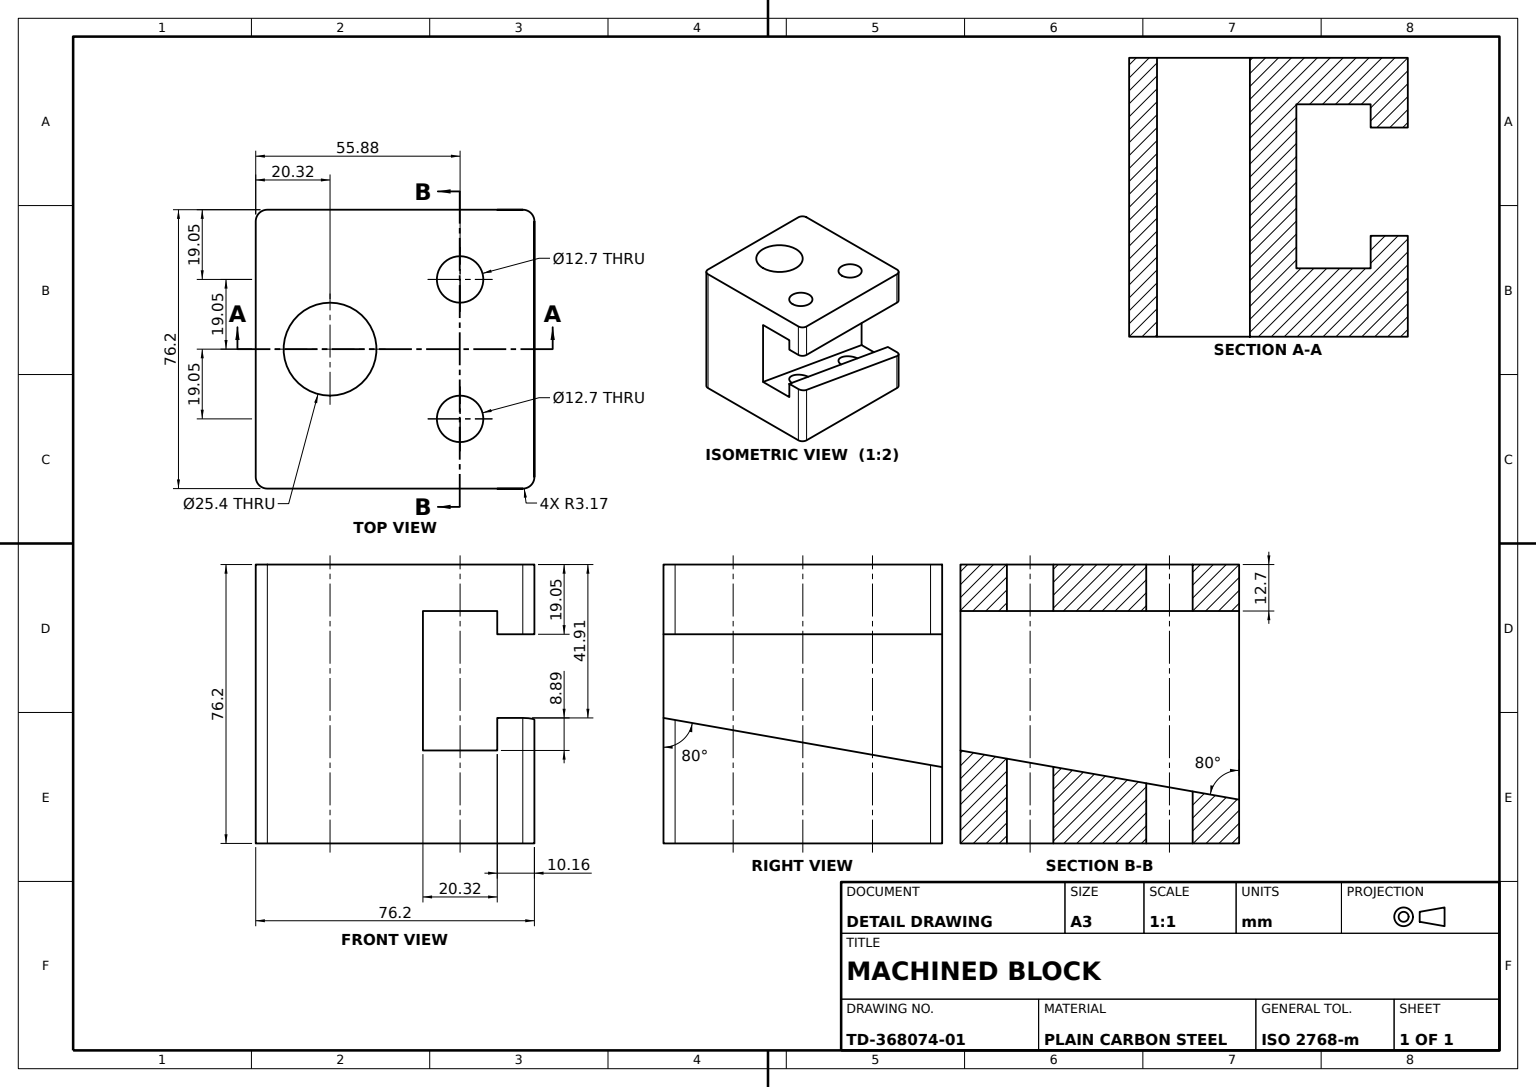
SolidWorks part; units mm, degrees
material "Plain Carbon Steel"
ref_plane "Front Plane" through (0, 0, 0) normal (0, 0, 1) x (1, 0, 0)
ref_plane "Top Plane" through (0, 0, 0) normal (0, 1, 0) x (1, 0, 0)
ref_plane "Right Plane" through (0, 0, 0) normal (1, 0, 0) x (0, 0, -1)
sketch "Block Profile Sketch" plane through (0, 0, 0) normal (0, 0, 1) x (1, 0, 0)
  line L1 (-38.1, -38.1) -> (38.1, -38.1)
  line L2 (-38.1, -38.1) -> (-38.1, 38.1)
  line L3 (-38.1, 38.1) -> (38.1, 38.1)
  line L4 (38.1, -38.1) -> (38.1, 38.1)
  line L5 (-38.1, -38.1) -> (38.1, 38.1) construction
  line L6 (-38.1, 38.1) -> (38.1, -38.1) construction
  point P0 (0, 0)
  dimension "D1" = 76.2
  dimension "D2" = 76.2
extrude "Block Body 3in" add sketch "Block Profile Sketch" along normal mid plane 76.2
sketch "Angled Slot Sketch" plane through (-38.1, 0, 0) normal (-1, 0, 0) x (0, 0, 1)
  line L0 (38.1, -17.2461) -> (-38.1, -3.81)
  line L1 (38.1, 38.1) -> (38.1, -38.1) construction
  line L2 (-38.1, 38.1) -> (-38.1, -38.1) construction
  line L3 (38.1, 38.1) -> (-38.1, 38.1) construction
  line L4 (38.1, -38.1) -> (-38.1, -38.1) construction
  line L5 (-38.1, -3.81) -> (-38.1, 19.05)
  line L6 (-38.1, 19.05) -> (38.1, 19.05)
  line L7 (38.1, 19.05) -> (38.1, -17.2461)
  dimension "D1" = 41.91
  dimension "D2" = 10
  dimension "D3" = 19.05
extrude "Angled Slot Cut" cut sketch "Angled Slot Sketch" against normal blind 10.16
sketch "Slot Undercut Sketch" plane through (-27.94, 0, 0) normal (-1, 0, 0) x (0, 0, 1)
  line L0 (-38.1, 25.4) -> (38.1, 25.4)
  line L1 (-38.1, 38.1) -> (-38.1, 19.05) construction
  line L2 (38.1, 38.1) -> (38.1, 19.05) construction
  line L3 (38.1, 25.4) -> (38.1, -26.1361)
  line L6 (-38.1, 19.05) -> (-38.1, -3.81) construction
  line L7 (-38.1, -12.7) -> (-38.1, 25.4)
  line L8 (38.1, 38.1) -> (-38.1, 38.1) construction
  line L10 (38.1, -26.1361) -> (-38.1, -12.7)
  dimension "D1" = 12.7
  dimension "D2" = 80
  dimension "D3" = 8.89
extrude "Slot Undercut Cut" cut sketch "Slot Undercut Sketch" against normal blind 20.32
fillet "Edge Fillets R0.125" radius 3.175 6 edges at (38.1, 0, -38.1) (-38.1, -20.955, -38.1) (-38.1, 28.575, -38.1) (38.1, 0, 38.1) (-38.1, -27.6731, 38.1) (-38.1, 28.575, 38.1)
sketch "Top Holes Sketch" plane through (0, 38.1, 0) normal (0, 1, 0) x (1, 0, 0)
  line L0 (34.925, 38.1) -> (-34.925, 38.1) construction
  line L1 (-38.1, -34.925) -> (-38.1, 34.925) construction
  line L2 (34.925, -38.1) -> (-34.925, -38.1) construction
  circle A0 centre (-17.78, 19.05) radius 6.35
  circle A1 centre (-17.78, -19.05) radius 6.35
  circle A2 centre (17.78, 0) radius 12.7
  dimension "D1" = 12.7
  dimension "D5" = 25.4
  dimension "D2" = 19.05
  dimension "D3" = 20.32
  dimension "D4" = 19.05
  dimension "D6" = 55.88
extrude "Top Holes 3x" cut sketch "Top Holes Sketch" against normal through all
